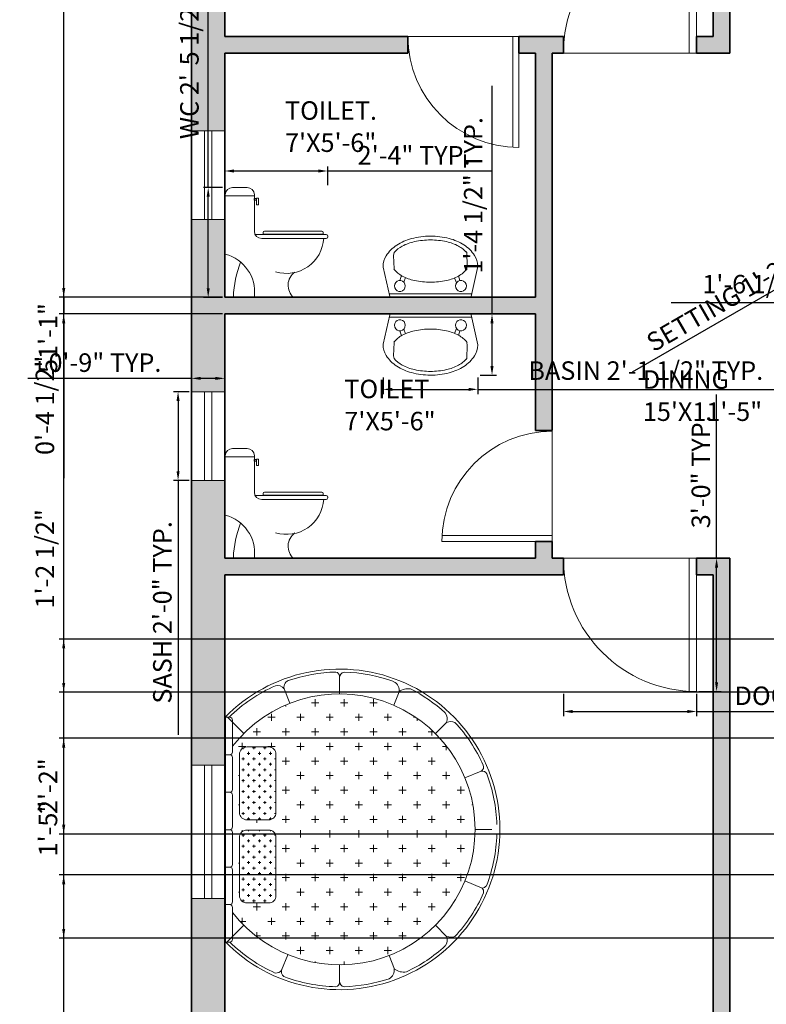
# Model space of a CAD drawing. Units: inches. Extents: x 2923 to 3500, y 1684 to 2381.
# Tile 2 of 12: x 2923 to 3125, y 1848 to 2114. Entities that reach past the tile are written whole.
import ezdxf

# ---------------------------------------------------------------- set-up
doc = ezdxf.new("R2010")
doc.units = ezdxf.units.IN
for name, color, linetype, lineweight in [('A-ANNO-DIMS', 2, 'Continuous', 18), ('A-AREA-IDEN', 7, 'Continuous', 18), ('A-DOOR', 3, 'Continuous', 18), ('A-FLOR-FIXT', 8, 'Continuous', 18), ('A-FURN-PATT', 8, 'Continuous', 13), ('A-GLAZ', 4, 'Continuous', 18), ('A-WALL', 7, 'Continuous', 35), ('A-WALL-PATT', 9, 'Continuous', 13), ('Furniture', 7, 'Continuous', 15)]:
    doc.layers.add(name, color=color, linetype=linetype, lineweight=lineweight)
doc.styles.get("Standard").update_dxf_attribs({"font": 'txt', "height": 5})
doc.dimstyles.new('ISO-25', dxfattribs={"dimtxt": 5, "dimasz": 2.5, "dimexe": 1.25, "dimexo": 0.625, "dimtad": 1, "dimlunit": 3, "dimtxsty": 'Standard', "dimcen": 2.5, "dimadec": 0, "dimazin": 0, "dimtfac": 1, "dimtmove": 0, "dimatfit": 3, "dimfxl": 1, "dimarcsym": 0})

# ---------------------------------------------------------------- blocks, each defined once
blk = doc.blocks.new('DOOR-SINGLE-36IN')
for p, q in [((36, 36), (0, 36)), ((34, 0.06), (34, 36)), ((36, 0), (36, 36))]:
    blk.add_line(p, q)
blk.add_arc((36, 36), 36, 180, 270)
blk = doc.blocks.new('DOOR-SINGLE-30IN')
for p, q in [((0, 30), (0, 0)), ((1.67, 29.95), (1.67, 0)), ((0, 0), (30, 0))]:
    blk.add_line(p, q)
blk.add_arc((0, 0), 30, 0, 90)
blk = doc.blocks.new('WINDOW-36IN')
for p, q in [((36, 9), (0, 9)), ((0, 9), (0, 0)), ((36, 0), (36, 9)), ((36, 5.5), (0, 5.5)), ((36, 3.5), (0, 3.5)), ((0, 0), (36, 0))]:
    blk.add_line(p, q)
blk = doc.blocks.new('WINDOW-24IN')
for p, q in [((9, 24), (0, 24)), ((0, 24), (0, 0)), ((3.5, 0), (3.5, 24)), ((5.5, 0), (5.5, 24)), ((9, 0), (9, 24)), ((0, 0), (9, 0))]:
    blk.add_line(p, q)
blk = doc.blocks.new('WC-FLOOR-MOUNT')
for p, q in [((6.05, 29.7), (2.11, 29.7)), ((0, 27.6), (0, 11.63)), ((7.97, 27.41), (0.2, 27.41)), ((8.49, 26.69), (7.97, 26.69)), ((7.97, 26.69), (7.97, 26.28)), ((8.02, 27.73), (8.02, 17.89)), ((8.02, 26.69), (8.02, 26.28)), ((8.49, 26.28), (8.49, 26.69)), ((9.1, 26.79), (8.59, 26.79)), ((8.59, 26.79), (8.59, 25.06)), ((9.1, 25.06), (9.1, 26.79)), ((7.97, 26.28), (8.49, 26.28)), ((8.59, 25.06), (9.1, 25.06)), ((27.42, 16.99), (8.24, 16.99)), ((10.4, 17.5), (10.4, 17.11)), ((10.4, 17.11), (26.62, 17.11)), ((26.23, 17.89), (10.79, 17.89)), ((15.89, 17.11), (15.89, 16.99)), ((23.77, 17.11), (23.77, 16.99)), ((26.62, 17.11), (26.62, 17.5)), ((27.82, 16.6), (27.82, 16.32)), ((27.42, 15.92), (9.99, 15.92)), ((8.02, 2.66), (8.02, 0.17)), ((8.02, 2.66), (8.02, 0.17)), ((18.71, 0.04), (2.25, 0.04))]:
    blk.add_line(p, q)
for centre, radius, start, end in [((2.11, 27.73), 1.97, 90, 180), ((6.05, 27.73), 1.97, 0, 90), ((9.99, 17.89), 1.97, 180, 270), ((10.79, 17.5), 0.394, 90, 180), ((16.71, 16.55), 10.05, 252.943, 356.7365), ((26.23, 17.5), 0.394, 0, 90), ((27.42, 16.6), 0.394, 0, 90), ((27.42, 16.32), 0.394, 270, 0), ((-2.41, 1.48), 10.5, 353.9182, 75.9043), ((31.43, -1.03), 29.12, 158.693, 177.6281), ((21.51, 3.3), 4.38, 125.5613, 228.8008)]:
    blk.add_arc(centre, radius, start, end)
blk = doc.blocks.new('BASIN-WALL-MOUNT')
for p, q in [((0, 8.4), (1.8, 16.33)), ((1.8, 16.54), (23.79, 16.54)), ((1.8, 16.13), (1.8, 16.54)), ((23.79, 16.54), (23.79, 16.13)), ((25.59, 8.23), (23.79, 16.33)), ((23.79, 15.64), (1.8, 15.64)), ((3.16, 14), (3.07, 13.48)), ((3.07, 13.48), (3.16, 12.95)), ((3.42, 14.46), (3.16, 14)), ((3.81, 14.8), (3.42, 14.46)), ((4.29, 14.98), (3.81, 14.8)), ((4.8, 14.98), (4.29, 14.98)), ((5.28, 14.8), (4.8, 14.98)), ((5.67, 14.46), (5.28, 14.8)), ((5.93, 14), (5.67, 14.46)), ((6.02, 13.48), (5.93, 14)), ((5.93, 12.95), (6.02, 13.48)), ((19.66, 14), (19.57, 13.48)), ((19.57, 13.48), (19.66, 12.95)), ((19.92, 14.46), (19.66, 14)), ((20.31, 14.8), (19.92, 14.46)), ((20.79, 14.98), (20.31, 14.8)), ((21.3, 14.98), (20.79, 14.98)), ((21.78, 14.8), (21.3, 14.98)), ((22.17, 14.46), (21.78, 14.8)), ((22.43, 14), (22.17, 14.46)), ((22.52, 13.48), (22.43, 14)), ((22.43, 12.95), (22.52, 13.48)), ((3.16, 12.95), (3.42, 12.49)), ((3.42, 12.49), (3.81, 12.15)), ((3.81, 12.15), (4.29, 11.97)), ((4.29, 11.97), (4.8, 11.97)), ((4.57, 11.96), (5.01, 10.67)), ((4.8, 11.97), (5.28, 12.15)), ((5.28, 12.15), (5.67, 12.49)), ((5.62, 12.45), (6.09, 11.17)), ((5.67, 12.49), (5.93, 12.95)), ((19.86, 12.63), (19.34, 11.26)), ((19.66, 12.95), (19.92, 12.49)), ((19.92, 12.49), (20.31, 12.15)), ((20.31, 12.15), (20.79, 11.97)), ((20.73, 11.97), (20.4, 10.75)), ((20.79, 11.97), (21.3, 11.97)), ((21.3, 11.97), (21.78, 12.15)), ((21.78, 12.15), (22.17, 12.49)), ((22.17, 12.49), (22.43, 12.95)), ((2.96, 8.83), (2.86, 5.21)), ((2.97, 8.99), (2.96, 8.98)), ((2.96, 8.98), (2.96, 8.97)), ((2.96, 8.97), (2.96, 8.96)), ((2.96, 8.83), (2.96, 8.96)), ((3.06, 9.08), (2.97, 8.99)), ((22.6, 4.46), (22.76, 8.08)), ((22.76, 8.08), (22.64, 8.8)), ((2.86, 5.21), (2.99, 4.47)), ((3.04, 4.25), (3.04, 4.25)), ((22.54, 4.2), (22.57, 4.35))]:
    blk.add_line(p, q)
for centre, radius, start, end in [((8.91, 3.89), 7.83, 118.2302, 139.6822), ((11.35, -0.82), 13.14, 102.6999, 117.8694), ((12.88, -8.38), 20.85, 90.2298, 102.2344), ((12.71, -8.38), 20.85, 77.7656, 89.7702), ((14.24, -0.82), 13.14, 62.1306, 77.3001), ((16.68, 3.89), 7.83, 39.3299, 61.7657), ((5.18, 8.21), 5.18, 177.9266, 179.8113), ((5.16, 8.15), 5.16, 179.1785, 213.1413), ((20.43, 8.08), 5.16, 326.4084, 0.3713), ((20.42, 8.14), 5.18, 359.7541, 0.9471), ((8.97, 10.54), 9.66, 212.6461, 237.0936), ((8.91, 9.59), 7.83, 220.8964, 241.7723), ((11.35, 14.31), 13.14, 242.1306, 257.3001), ((14.24, 14.31), 13.14, 282.6999, 297.8694), ((16.68, 9.59), 7.83, 298.2281, 319.1983), ((16.64, 10.51), 9.66, 302.4413, 326.8887), ((11.42, 14.45), 14.27, 237.383, 254.6821), ((12.95, 20.75), 20.75, 255.1956, 269.4863), ((12.88, 21.87), 20.85, 257.7656, 269.7702), ((12.75, 20.75), 20.75, 270.0316, 284.3223), ((12.71, 21.87), 20.85, 270.2298, 282.2344), ((14.23, 14.44), 14.27, 284.841, 302.14)]:
    blk.add_arc(centre, radius, start, end)
blk = doc.blocks.new('BED-ROUND-FRAME')
for p, q in [((31.04, 79.92), (31.04, 84.58)), ((31.04, 79.92), (31.04, 84.58)), ((17.61, 77.37), (16.05, 81.29)), ((45.66, 76.84), (47.11, 80.49)), ((0, 13.11), (0, 73.51)), ((5.15, 69.2), (0.74, 73.61)), ((5.15, 69.2), (0.74, 73.61)), ((56.93, 69.2), (59.95, 72.21)), ((56.93, 69.2), (59.95, 72.21)), ((59.95, 72.21), (56.93, 69.2)), ((13.83, 63.84), (13.83, 47.62)), ((64.9, 57.24), (69.31, 59.05)), ((69.31, 59.05), (69.4, 59.09)), ((67.65, 43.31), (72.18, 43.31)), ((13.83, 41.4), (13.83, 25.18)), ((13.83, 39.13), (13.84, 39.12)), ((64.9, 29.37), (69.53, 27.47)), ((0.42, 12.68), (5.15, 17.42)), ((0.42, 12.68), (5.15, 17.42)), ((59.95, 14.4), (56.93, 17.42)), ((17.07, 9.46), (15.35, 5.25)), ((44.42, 9.23), (45.86, 5.58)), ((31.04, 1.98), (31.04, 6.69)), ((31.04, 2.04), (31.04, 6.69))]:
    blk.add_line(p, q)
for points in [[(4, 47.85), (4, 63.6, -0.414214), (5.97, 65.57), (11.88, 65.57, -0.414214), (13.84, 63.6), (13.84, 47.85, -0.414214), (11.88, 45.89), (5.97, 45.89, -0.414214)], [(4, 25.41), (4, 41.16, -0.414214), (5.97, 43.13), (11.88, 43.13, -0.414214), (13.84, 41.16), (13.84, 25.41, -0.414214), (11.88, 23.45), (5.97, 23.45, -0.414214)]]:
    blk.add_lwpolyline(points, format="xyb", close=True)
for centre, radius, start, end in [((31.04, 43.31), 43.31, 224.213, 135.787), ((31.04, 43.31), 42.52, 91.3819, 109.0292), ((29.76, 84.56), 1.29, 359.0498, 78.348), ((32.5, 84.36), 1.46, 98.688, 183.9778), ((31.04, 43.31), 42.52, 69.8397, 88.3303), ((17.88, 81.76), 1.88, 111.9527, 202.5488), ((44.67, 80.98), 2.46, 345.7709, 65.4979), ((31.04, 43.31), 42.52, 114.0695, 134.5949), ((31.04, 43.31), 36.61, 217.8198, 142.1802), ((14.23, 79.9), 2.29, 37.3562, 103.3498), ((49.64, 77.03), 4.29, 82.908, 126.1659), ((31.04, 43.31), 42.52, 47.802, 63.2705), ((57.53, 73.21), 2.61, 337.5919, 37.6583), ((61.1, 69.09), 3.33, 70.4217, 110.1689), ((31.04, 43.31), 42.52, 24.0703, 42.854), ((69.6, 57.73), 1.36, 26.1665, 102.6069), ((68.6, 60.18), 1.35, 304.4266, 20.4145), ((31.04, 43.31), 42.52, 1.7281, 20.7271), ((31.04, 43.31), 42.52, 339.0428, 358.2719), ((69.4, 29.21), 1.75, 274.2316, 320.4352), ((68.35, 26.36), 1.62, 353.6066, 43.1756), ((31.04, 43.31), 42.52, 317.146, 336.245), ((57.53, 13.4), 2.61, 322.3417, 22.4081), ((61.1, 17.52), 3.33, 249.8311, 289.5783), ((31.04, 43.31), 42.52, 225.7269, 245.8957), ((31.04, 43.31), 42.52, 295.113, 312.198), ((16.89, 4.85), 1.59, 153.9459, 235.5493), ((42.79, 5.51), 3.04, 302.4304, 3.4261), ((48.39, 9.04), 4.29, 233.8341, 279.2916), ((13.85, 6.32), 1.83, 264.4179, 326.0029), ((31.04, 43.31), 42.52, 249.2703, 268.6181), ((31.04, 43.31), 42.52, 271.6697, 288.3347), ((29.76, 2.06), 1.29, 281.652, 0.9502), ((32.5, 2.25), 1.46, 176.0222, 261.312)]:
    blk.add_arc(centre, radius, start, end)
blk = doc.blocks.new('*D23')
at = {"layer": 'A-ANNO-DIMS', "color": 0, "lineweight": -2, "transparency": 16777216}
for p, q in [((2968.6, 2013.41), (2964.38, 2013.41)), ((2965.63, 2010.91), (2965.63, 1991.91)), ((2968.6, 1989.41), (2964.38, 1989.41)), ((2965.63, 1989.41), (2965.63, 1920.66))]:
    blk.add_line(p, q, dxfattribs=at)
at = {"layer": 'A-ANNO-DIMS', "color": 0, "transparency": 16777216}
for points in [[(2965.21, 2010.91), (2966.05, 2010.91), (2965.63, 2013.41)], [(2965.21, 1991.91), (2966.05, 1991.91), (2965.63, 1989.41)]]:
    blk.add_solid(points, dxfattribs=at)
at = {"layer": 'Defpoints', "color": 0, "transparency": 16777216}
for p in [(2969.23, 2013.41), (2965.63, 1989.41), (2969.23, 1989.41)]:
    blk.add_point(p, dxfattribs=at)
at = {"layer": 'A-ANNO-DIMS', "color": 0, "transparency": 16777216, "insert": (2962.03, 1953.78), "char_height": 5, "attachment_point": 5, "rotation": 90}
blk.add_mtext('SASH 2\'-0" TYP.', dxfattribs=at)
blk = doc.blocks.new('*D24')
at = {"layer": 'A-ANNO-DIMS', "color": 0, "lineweight": -2, "transparency": 16777216}
for p, q in [((2969.23, 2017.01), (2925, 2017.01)), ((2969.23, 2014.03), (2969.23, 2018.26)), ((2975.73, 2017.01), (2971.73, 2017.01)), ((2978.23, 2014.03), (2978.23, 2018.26))]:
    blk.add_line(p, q, dxfattribs=at)
at = {"layer": 'A-ANNO-DIMS', "color": 0, "transparency": 16777216}
for points in [[(2971.73, 2017.42), (2971.73, 2016.59), (2969.23, 2017.01)], [(2975.73, 2017.42), (2975.73, 2016.59), (2978.23, 2017.01)]]:
    blk.add_solid(points, dxfattribs=at)
at = {"layer": 'Defpoints', "color": 0, "transparency": 16777216}
for p in [(2969.23, 2017.01), (2969.23, 2013.41), (2978.23, 2013.41)]:
    blk.add_point(p, dxfattribs=at)
at = {"layer": 'A-ANNO-DIMS', "color": 0, "transparency": 16777216, "insert": (2945.87, 2020.61), "char_height": 5, "attachment_point": 5}
blk.add_mtext('0\'-9" TYP.', dxfattribs=at)
blk = doc.blocks.new('*D25')
at = {"layer": 'A-ANNO-DIMS', "color": 0, "lineweight": -2, "transparency": 16777216}
for p, q in [((3069.73, 1931.78), (3069.73, 1925.76)), ((3105.73, 1931.78), (3105.73, 1925.76)), ((3072.23, 1927.01), (3103.23, 1927.01)), ((3105.73, 1927.01), (3174.96, 1927.01))]:
    blk.add_line(p, q, dxfattribs=at)
at = {"layer": 'A-ANNO-DIMS', "color": 0, "transparency": 16777216}
for points in [[(3072.23, 1927.42), (3072.23, 1926.59), (3069.73, 1927.01)], [(3103.23, 1927.42), (3103.23, 1926.59), (3105.73, 1927.01)]]:
    blk.add_solid(points, dxfattribs=at)
at = {"layer": 'Defpoints', "color": 0, "transparency": 16777216}
for p in [(3069.73, 1932.41), (3105.73, 1932.41), (3105.73, 1927.01)]:
    blk.add_point(p, dxfattribs=at)
at = {"layer": 'A-ANNO-DIMS', "color": 0, "transparency": 16777216, "insert": (3141.59, 1930.61), "char_height": 5, "attachment_point": 5}
blk.add_mtext('DOOR 3\'-0" TYP.', dxfattribs=at)
blk = doc.blocks.new('*D26')
at = {"layer": 'A-ANNO-DIMS', "color": 0, "lineweight": -2, "transparency": 16777216}
for p, q in [((3111.13, 1968.41), (3111.13, 2012.63)), ((3106.35, 1968.41), (3112.38, 1968.41)), ((3111.13, 1934.91), (3111.13, 1965.91)), ((3106.35, 1932.41), (3112.38, 1932.41))]:
    blk.add_line(p, q, dxfattribs=at)
at = {"layer": 'A-ANNO-DIMS', "color": 0, "transparency": 16777216}
for points in [[(3110.71, 1965.91), (3111.55, 1965.91), (3111.13, 1968.41)], [(3110.71, 1934.91), (3111.55, 1934.91), (3111.13, 1932.41)]]:
    blk.add_solid(points, dxfattribs=at)
at = {"layer": 'Defpoints', "color": 0, "transparency": 16777216}
for p in [(3105.73, 1968.41), (3111.13, 1968.41), (3105.73, 1932.41)]:
    blk.add_point(p, dxfattribs=at)
at = {"layer": 'A-ANNO-DIMS', "color": 0, "transparency": 16777216, "insert": (3107.53, 1991.77), "char_height": 5, "attachment_point": 5, "rotation": 90}
blk.add_mtext('3\'-0" TYP.', dxfattribs=at)
blk = doc.blocks.new('*D35')
at = {"layer": 'A-ANNO-DIMS', "color": 0, "lineweight": -2, "transparency": 16777216}
for p, q in [((2973.77, 2068.57), (2973.77, 2146.37)), ((2977.6, 2068.57), (2972.52, 2068.57)), ((2973.77, 2041.37), (2973.77, 2066.07)), ((2977.6, 2038.87), (2972.52, 2038.87))]:
    blk.add_line(p, q, dxfattribs=at)
at = {"layer": 'A-ANNO-DIMS', "color": 0, "transparency": 16777216}
for points in [[(2973.36, 2066.07), (2974.19, 2066.07), (2973.77, 2068.57)], [(2973.36, 2041.37), (2974.19, 2041.37), (2973.77, 2038.87)]]:
    blk.add_solid(points, dxfattribs=at)
at = {"layer": 'Defpoints', "color": 0, "transparency": 16777216}
for p in [(2973.77, 2068.57), (2978.23, 2068.57), (2978.23, 2038.87)]:
    blk.add_point(p, dxfattribs=at)
at = {"layer": 'A-ANNO-DIMS', "color": 0, "transparency": 16777216, "insert": (2969.34, 2108.72), "char_height": 5, "attachment_point": 5, "rotation": 90}
blk.add_mtext('WC 2\'-5 1/2" TYP.', dxfattribs=at)
blk = doc.blocks.new('*D36')
at = {"layer": 'A-ANNO-DIMS', "color": 0, "lineweight": -2, "transparency": 16777216}
for p, q in [((2978.23, 2069.2), (2978.23, 2074.28)), ((2980.73, 2073.03), (3003.55, 2073.03)), ((3006.05, 2069.2), (3006.05, 2074.28)), ((3006.05, 2073.03), (3050.27, 2073.03))]:
    blk.add_line(p, q, dxfattribs=at)
at = {"layer": 'A-ANNO-DIMS', "color": 0, "transparency": 16777216}
for points in [[(2980.73, 2073.44), (2980.73, 2072.61), (2978.23, 2073.03)], [(3003.55, 2073.44), (3003.55, 2072.61), (3006.05, 2073.03)]]:
    blk.add_solid(points, dxfattribs=at)
at = {"layer": 'Defpoints', "color": 0, "transparency": 16777216}
for p in [(3006.05, 2073.03), (2978.23, 2068.57), (3006.05, 2068.57)]:
    blk.add_point(p, dxfattribs=at)
at = {"layer": 'A-ANNO-DIMS', "color": 0, "transparency": 16777216, "insert": (3029.41, 2076.63), "char_height": 5, "attachment_point": 5}
blk.add_mtext('2\'-4" TYP.', dxfattribs=at)
blk = doc.blocks.new('*D37')
at = {"layer": 'A-ANNO-DIMS', "color": 0, "lineweight": -2, "transparency": 16777216}
for p, q in [((3021, 2017.25), (3021, 2012.78)), ((3046.61, 2017.25), (3046.61, 2012.78)), ((3023.5, 2014.03), (3044.11, 2014.03)), ((3046.61, 2014.03), (3134.88, 2014.03))]:
    blk.add_line(p, q, dxfattribs=at)
at = {"layer": 'A-ANNO-DIMS', "color": 0, "transparency": 16777216}
for points in [[(3023.5, 2014.45), (3023.5, 2013.61), (3021, 2014.03)], [(3044.11, 2014.45), (3044.11, 2013.61), (3046.61, 2014.03)]]:
    blk.add_solid(points, dxfattribs=at)
at = {"layer": 'Defpoints', "color": 0, "transparency": 16777216}
for p in [(3021, 2017.87), (3046.61, 2017.87), (3046.61, 2014.03)]:
    blk.add_point(p, dxfattribs=at)
at = {"layer": 'A-ANNO-DIMS', "color": 0, "transparency": 16777216, "insert": (3092, 2018.46), "char_height": 5, "attachment_point": 5}
blk.add_mtext('BASIN 2\'-1 1/2" TYP.', dxfattribs=at)
blk = doc.blocks.new('*D38')
at = {"layer": 'A-ANNO-DIMS', "color": 0, "lineweight": -2, "transparency": 16777216}
for p, q in [((3050.45, 2034.41), (3050.45, 2096.01)), ((3047.23, 2034.41), (3051.7, 2034.41)), ((3050.45, 2020.37), (3050.45, 2031.91)), ((3047.23, 2017.87), (3051.7, 2017.87))]:
    blk.add_line(p, q, dxfattribs=at)
at = {"layer": 'A-ANNO-DIMS', "color": 0, "transparency": 16777216}
for points in [[(3050.03, 2031.91), (3050.87, 2031.91), (3050.45, 2034.41)], [(3050.03, 2020.37), (3050.87, 2020.37), (3050.45, 2017.87)]]:
    blk.add_solid(points, dxfattribs=at)
at = {"layer": 'Defpoints', "color": 0, "transparency": 16777216}
for p in [(3046.61, 2034.41), (3050.45, 2034.41), (3046.61, 2017.87)]:
    blk.add_point(p, dxfattribs=at)
at = {"layer": 'A-ANNO-DIMS', "color": 0, "transparency": 16777216, "insert": (3046.02, 2066.46), "char_height": 5, "attachment_point": 5, "rotation": 90}
blk.add_mtext('1\'-4 1/2" TYP.', dxfattribs=at)
blk = doc.blocks.new('*D40')
at = {"layer": 'A-ANNO-DIMS', "color": 0, "lineweight": -2, "transparency": 16777216}
for p, q in [((3160.47, 2034.91), (3160.47, 2038.63)), ((3178.95, 2034.91), (3178.95, 2038.63)), ((3160.47, 2037.38), (3098.86, 2037.38)), ((3176.45, 2037.38), (3162.97, 2037.38))]:
    blk.add_line(p, q, dxfattribs=at)
at = {"layer": 'A-ANNO-DIMS', "color": 0, "transparency": 16777216}
for points in [[(3162.97, 2037.8), (3162.97, 2036.96), (3160.47, 2037.38)], [(3176.45, 2037.8), (3176.45, 2036.96), (3178.95, 2037.38)]]:
    blk.add_solid(points, dxfattribs=at)
at = {"layer": 'Defpoints', "color": 0, "transparency": 16777216}
for p in [(3160.47, 2037.38), (3160.47, 2034.29), (3178.95, 2034.29)]:
    blk.add_point(p, dxfattribs=at)
at = {"layer": 'A-ANNO-DIMS', "color": 0, "transparency": 16777216, "insert": (3128.42, 2041.81), "char_height": 5, "attachment_point": 5}
blk.add_mtext('1\'-6 1/2" TYP.', dxfattribs=at)
blk = doc.blocks.new('*D41')
at = {"layer": 'A-ANNO-DIMS', "color": 0, "lineweight": -2, "transparency": 16777216}
for p, q in [((3166.89, 2065.67), (3168.23, 2063.34)), ((3165.44, 2063.18), (3157.85, 2058.8)), ((3155.69, 2057.55), (3088.31, 2018.65)), ((3154.97, 2058.79), (3156.31, 2056.46))]:
    blk.add_line(p, q, dxfattribs=at)
at = {"layer": 'A-ANNO-DIMS', "color": 0, "transparency": 16777216}
for points in [[(3165.23, 2063.54), (3165.65, 2062.82), (3167.61, 2064.43)], [(3157.64, 2059.16), (3158.06, 2058.43), (3155.69, 2057.55)]]:
    blk.add_solid(points, dxfattribs=at)
at = {"layer": 'Defpoints', "color": 0, "transparency": 16777216}
for p in [(3166.57, 2066.21), (3154.66, 2059.33), (3155.69, 2057.55)]:
    blk.add_point(p, dxfattribs=at)
at = {"layer": 'A-ANNO-DIMS', "color": 0, "transparency": 16777216, "insert": (3119.12, 2040.59), "char_height": 5, "attachment_point": 5, "rotation": 30}
blk.add_mtext('SETTING 1\'-2" TYP.', dxfattribs=at)
blk = doc.blocks.new('*D49')
at = {"layer": 'A-ANNO-DIMS', "color": 0, "lineweight": -2, "transparency": 16777216}
for p, q in [((2969.23, 2263.03), (2969.23, 2370.16)), ((3444.23, 2110.03), (3444.23, 2370.16)), ((2971.73, 2368.91), (3441.73, 2368.91))]:
    blk.add_line(p, q, dxfattribs=at)
at = {"layer": 'A-ANNO-DIMS', "color": 0, "transparency": 16777216}
for points in [[(2971.73, 2369.32), (2971.73, 2368.49), (2969.23, 2368.91)], [(3441.73, 2369.32), (3441.73, 2368.49), (3444.23, 2368.91)]]:
    blk.add_solid(points, dxfattribs=at)
at = {"layer": 'Defpoints', "color": 0, "transparency": 16777216}
for p in [(3444.23, 2368.91), (2969.23, 2262.41), (3444.23, 2109.41)]:
    blk.add_point(p, dxfattribs=at)
at = {"layer": 'A-ANNO-DIMS', "color": 0, "transparency": 16777216, "insert": (3206.73, 2372.51), "char_height": 5, "attachment_point": 5}
blk.add_mtext('39\'-7"', dxfattribs=at)
blk = doc.blocks.new('*D50')
at = {"layer": 'A-ANNO-DIMS', "color": 0, "lineweight": -2, "transparency": 16777216}
for p, q in [((2991.1, 2334.41), (2933.48, 2334.41)), ((2934.73, 1723.91), (2934.73, 2331.91)), ((3109.6, 1721.41), (2933.48, 1721.41))]:
    blk.add_line(p, q, dxfattribs=at)
at = {"layer": 'A-ANNO-DIMS', "color": 0, "transparency": 16777216}
for points in [[(2934.31, 2331.91), (2935.15, 2331.91), (2934.73, 2334.41)], [(2934.31, 1723.91), (2935.15, 1723.91), (2934.73, 1721.41)]]:
    blk.add_solid(points, dxfattribs=at)
at = {"layer": 'Defpoints', "color": 0, "transparency": 16777216}
for p in [(2934.73, 2334.41), (2991.73, 2334.41), (3110.23, 1721.41)]:
    blk.add_point(p, dxfattribs=at)
at = {"layer": 'A-ANNO-DIMS', "color": 0, "transparency": 16777216, "insert": (2931.13, 2027.91), "char_height": 5, "attachment_point": 5, "rotation": 90}
blk.add_mtext('51\'-1"', dxfattribs=at)
blk = doc.blocks.new('*D51')
at = {"layer": 'A-ANNO-DIMS', "color": 0, "lineweight": -2, "transparency": 16777216}
for p, q in [((2934.73, 2041.41), (2934.73, 2043.91)), ((2977.6, 2038.91), (2933.48, 2038.91)), ((2934.73, 2038.91), (2934.73, 2034.41)), ((2977.6, 2034.41), (2933.48, 2034.41)), ((2934.73, 2031.91), (2934.73, 1990.06))]:
    blk.add_line(p, q, dxfattribs=at)
at = {"layer": 'A-ANNO-DIMS', "color": 0, "transparency": 16777216}
for points in [[(2934.31, 2041.41), (2935.15, 2041.41), (2934.73, 2038.91)], [(2934.31, 2031.91), (2935.15, 2031.91), (2934.73, 2034.41)]]:
    blk.add_solid(points, dxfattribs=at)
at = {"layer": 'Defpoints', "color": 0, "transparency": 16777216}
for p in [(2978.23, 2038.91), (2934.73, 2034.41), (2978.23, 2034.41)]:
    blk.add_point(p, dxfattribs=at)
at = {"layer": 'A-ANNO-DIMS', "color": 0, "transparency": 16777216, "insert": (2930.3, 2009.73), "char_height": 5, "attachment_point": 5, "rotation": 90}
blk.add_mtext('0\'-4 1/2"', dxfattribs=at)
blk = doc.blocks.new('*D63')
at = {"layer": 'A-ANNO-DIMS', "color": 0, "lineweight": -2, "transparency": 16777216}
for p, q in [((3203.71, 1919.77), (2933.48, 1919.77)), ((2934.73, 1896.41), (2934.73, 1917.27)), ((3203.71, 1893.91), (2933.48, 1893.91))]:
    blk.add_line(p, q, dxfattribs=at)
at = {"layer": 'A-ANNO-DIMS', "color": 0, "transparency": 16777216}
for points in [[(2934.31, 1917.27), (2935.15, 1917.27), (2934.73, 1919.77)], [(2934.31, 1896.41), (2935.15, 1896.41), (2934.73, 1893.91)]]:
    blk.add_solid(points, dxfattribs=at)
at = {"layer": 'Defpoints', "color": 0, "transparency": 16777216}
for p in [(2934.73, 1919.77), (3204.33, 1919.77), (3204.33, 1893.91)]:
    blk.add_point(p, dxfattribs=at)
at = {"layer": 'A-ANNO-DIMS', "color": 0, "transparency": 16777216, "insert": (2931.13, 1906.84), "char_height": 5, "attachment_point": 5, "rotation": 90}
blk.add_mtext('2\'-2"', dxfattribs=at)
blk = doc.blocks.new('*D65')
at = {"layer": 'A-ANNO-DIMS', "color": 0, "lineweight": -2, "transparency": 16777216}
for p, q in [((2934.73, 1882.85), (2934.73, 1905.41)), ((3193.07, 1882.85), (2933.48, 1882.85)), ((2934.73, 1868.29), (2934.73, 1880.35)), ((3193.07, 1865.79), (2933.48, 1865.79))]:
    blk.add_line(p, q, dxfattribs=at)
at = {"layer": 'A-ANNO-DIMS', "color": 0, "transparency": 16777216}
for points in [[(2934.31, 1880.35), (2935.15, 1880.35), (2934.73, 1882.85)], [(2934.31, 1868.29), (2935.15, 1868.29), (2934.73, 1865.79)]]:
    blk.add_solid(points, dxfattribs=at)
at = {"layer": 'Defpoints', "color": 0, "transparency": 16777216}
for p in [(2934.73, 1882.85), (3193.7, 1882.85), (3193.7, 1865.79)]:
    blk.add_point(p, dxfattribs=at)
at = {"layer": 'A-ANNO-DIMS', "color": 0, "transparency": 16777216, "insert": (2931.13, 1895.38), "char_height": 5, "attachment_point": 5, "rotation": 90}
blk.add_mtext('1\'-5"', dxfattribs=at)
blk = doc.blocks.new('*D67')
at = {"layer": 'A-ANNO-DIMS', "color": 0, "lineweight": -2, "transparency": 16777216}
for p, q in [((2934.73, 1946.56), (2934.73, 1987.45)), ((3208.37, 1946.56), (2933.48, 1946.56)), ((2934.73, 1934.74), (2934.73, 1944.06)), ((3208.37, 1932.24), (2933.48, 1932.24))]:
    blk.add_line(p, q, dxfattribs=at)
at = {"layer": 'A-ANNO-DIMS', "color": 0, "transparency": 16777216}
for points in [[(2934.31, 1944.06), (2935.15, 1944.06), (2934.73, 1946.56)], [(2934.31, 1934.74), (2935.15, 1934.74), (2934.73, 1932.24)]]:
    blk.add_solid(points, dxfattribs=at)
at = {"layer": 'Defpoints', "color": 0, "transparency": 16777216}
for p in [(2934.73, 1946.56), (3209, 1946.56), (3209, 1932.24)]:
    blk.add_point(p, dxfattribs=at)
at = {"layer": 'A-ANNO-DIMS', "color": 0, "transparency": 16777216, "insert": (2930.3, 1968.26), "char_height": 5, "attachment_point": 5, "rotation": 90}
blk.add_mtext('1\'-2 1/2"', dxfattribs=at)

msp = doc.modelspace()

# ---------------------------------------------------------------- hatches: boundary and pattern name
at = {"layer": 'A-FURN-PATT'}
h = msp.add_hatch(dxfattribs=at)
h.set_pattern_fill('CROSS', color=256, scale=15.748, angle=180, style=0)
h.set_pattern_definition([(360, (1245.7636, 386.063), (3.937, -3.937), [1.9685, -5.9055]), (270, (1246.748, 387.0473), (-3.937, -3.937), [1.9685, -5.9055])])
h.paths.add_polyline_path([(2980.347, 1917.607), (2980.347, 1915.314), (2979.599, 1915.314, -0.4142136), (2980.347, 1914.565), (2980.347, 1905.193), (2979.599, 1905.193, -0.4142136), (2980.347, 1904.445), (2980.347, 1895.073), (2979.599, 1895.073, -0.4142136), (2980.347, 1894.325), (2980.347, 1884.952), (2979.599, 1884.952, -0.4142136), (2980.347, 1884.204), (2980.347, 1874.832), (2979.599, 1874.832, -0.4142136), (2980.347, 1874.084), (2980.347, 1872.705, 2.9191153)])
h.paths.add_polyline_path([(2992.074, 1877.263, -0.4142136), (2990.105, 1875.294), (2984.2, 1875.294, -0.4142136), (2982.231, 1877.263), (2982.231, 1893.011, -0.4142136), (2984.2, 1894.979), (2990.105, 1894.979, -0.4142136), (2992.074, 1893.011)], flags=16)
h.paths.add_polyline_path([(2992.074, 1899.703, -0.4142136), (2990.105, 1897.735), (2984.2, 1897.735, -0.4142136), (2982.231, 1899.703), (2982.231, 1915.451, -0.4142136), (2984.2, 1917.42), (2990.105, 1917.42, -0.4142136), (2992.074, 1915.451)], flags=16)
h = msp.add_hatch(dxfattribs=at)
h.set_pattern_fill('CROSS', color=256, scale=5.9055, angle=450, style=0)
h.set_pattern_definition([(90, (3722.8477, 1218.4861), (-1.476375, 1.476375), [0.7381875, -2.2145625]), (180, (3723.2168, 1218.8552), (-1.476375, -1.476375), [0.7381875, -2.2145625])])
h.paths.add_polyline_path([(2982.231, 1877.263, 0.4142136), (2984.2, 1875.294), (2990.105, 1875.294, 0.4142136), (2992.074, 1877.263), (2992.074, 1893.011, 0.4142136), (2990.105, 1894.979), (2984.2, 1894.979, 0.4142136), (2982.231, 1893.011)])
h.paths.add_polyline_path([(2992.074, 1915.451, 0.4142136), (2990.105, 1917.42), (2984.2, 1917.42, 0.4142136), (2982.231, 1915.451), (2982.231, 1899.703, 0.4142136), (2984.2, 1897.735), (2990.105, 1897.735, 0.4142136), (2992.074, 1899.703)])
at = {"layer": 'A-WALL-PATT'}
h = msp.add_hatch(color=256, dxfattribs=at)
h.dxf.hatch_style = 1
h.paths.add_polyline_path([(3014.23, 2262.406), (2969.23, 2262.406), (2969.23, 2201.5), (2978.23, 2201.5), (2978.23, 2213.699), (2978.23, 2253.406), (3014.23, 2253.406)])
h.paths.add_polyline_path([(3119.23, 2262.406), (3074.23, 2262.406), (3074.23, 2253.406), (3110.23, 2253.406), (3110.23, 2109.406), (3105.73, 2109.406), (3105.73, 2104.906), (3114.73, 2104.906), (3114.73, 2152.906), (3119.23, 2152.906), (3119.23, 2157.406), (3114.73, 2157.406), (3114.73, 2253.406), (3119.23, 2253.406)])
h.paths.add_polyline_path([(3179.98, 2262.406), (3149.23, 2262.406), (3149.23, 2253.406), (3179.98, 2253.406)], flags=0)
h.paths.add_polyline_path([(3295.73, 2262.406), (3215.98, 2262.406), (3215.98, 2253.406), (3246.73, 2253.406), (3246.73, 2157.406), (3149.23, 2157.406), (3149.23, 2152.906), (3246.73, 2152.906), (3246.73, 2149.906), (3251.23, 2149.906), (3251.23, 2253.406), (3295.73, 2253.406)])
h.paths.add_polyline_path([(3397.23, 2262.406), (3343.73, 2262.406), (3343.73, 2253.406), (3349.929, 2253.406), (3388.23, 2253.406), (3388.23, 2199.406), (3397.23, 2199.406)])
h.paths.add_polyline_path([(3369.935, 2334.406), (3264.935, 2334.406), (3264.935, 2262.406), (3269.435, 2262.406), (3269.435, 2329.906), (3365.435, 2329.906), (3365.435, 2262.406), (3369.935, 2262.406)])
h.paths.add_polyline_path([(3096.73, 2334.406), (2991.73, 2334.406), (2991.73, 2262.406), (2996.23, 2262.406), (2996.23, 2329.906), (3092.23, 2329.906), (3092.23, 2262.406), (3096.73, 2262.406)])
h.paths.add_polyline_path([(3397.23, 2163.406), (3388.23, 2163.406), (3388.23, 2109.406), (3251.23, 2109.406), (3251.23, 2113.906), (3246.73, 2113.906), (3246.73, 2092.906), (3251.23, 2092.906), (3251.23, 2104.906), (3435.23, 2104.906), (3435.23, 2080.906), (3444.23, 2080.906), (3444.23, 2109.406), (3397.23, 2109.406)])
h.paths.add_polyline_path([(3444.23, 2044.906), (3435.23, 2044.906), (3435.23, 2020.906), (3251.23, 2020.906), (3251.23, 2032.906), (3246.73, 2032.906), (3246.73, 2016.406), (3251.23, 2016.406), (3287.73, 2016.406), (3287.73, 1968.406), (3287.23, 1968.406), (3287.23, 1963.906), (3296.73, 1963.906), (3296.73, 1968.406), (3292.23, 1968.406), (3292.23, 2016.406), (3388.23, 2016.406), (3388.23, 2004.398), (3397.23, 2004.398), (3397.23, 2016.406), (3444.23, 2016.406)])
h.paths.add_polyline_path([(3397.23, 1980.398), (3388.23, 1980.398), (3388.23, 1979.998), (3388.23, 1969.828), (3388.23, 1968.406), (3326.73, 1968.406), (3326.73, 1963.906), (3388.23, 1963.906), (3388.23, 1913.156), (3397.23, 1913.156)])
h.paths.add_polyline_path([(3251.23, 1968.406), (3150.73, 1968.406), (3150.73, 1963.906), (3246.73, 1963.906), (3246.73, 1826.406), (3230.98, 1826.406), (3230.98, 1817.406), (3251.23, 1817.406), (3251.23, 1963.906)])
h.paths.add_polyline_path([(3114.73, 1968.406), (3105.73, 1968.406), (3105.73, 1963.906), (3110.23, 1963.906), (3110.23, 1817.406), (3119.23, 1817.406), (3119.23, 1826.406), (3114.73, 1826.406)])
h.paths.add_polyline_path([(3069.73, 1968.406), (3066.73, 1968.406), (3066.73, 1972.906), (3062.23, 1972.906), (3062.23, 1968.406), (2978.23, 1968.406), (2978.23, 1989.406), (2969.23, 1989.406), (2969.23, 1912.505), (2978.23, 1912.505), (2978.23, 1925.355), (2978.23, 1963.906), (3069.73, 1963.906)])
h.paths.add_polyline_path([(3066.73, 2104.906), (3069.73, 2104.906), (3069.73, 2109.406), (3057.73, 2109.406), (3057.73, 2104.906), (3062.23, 2104.906), (3062.23, 2038.906), (2978.23, 2038.906), (2978.23, 2059.906), (2969.23, 2059.906), (2969.23, 2013.406), (2978.23, 2013.406), (2978.23, 2034.406), (3062.23, 2034.406), (3062.23, 2002.906), (3066.73, 2002.906)])
h.paths.add_polyline_path([(3027.73, 2109.406), (2978.23, 2109.406), (2978.23, 2165.5), (2969.23, 2165.5), (2969.23, 2083.906), (2978.23, 2083.906), (2978.23, 2104.906), (3027.73, 2104.906)])
h.paths.add_polyline_path([(2978.23, 1876.505), (2969.23, 1876.505), (2969.23, 1817.406), (3014.23, 1817.406), (3014.23, 1826.406), (2978.23, 1826.406)])
h.paths.add_polyline_path([(2996.23, 1817.406), (2991.73, 1817.406), (2991.73, 1745.406), (3096.73, 1745.406), (3096.73, 1817.406), (3092.23, 1817.406), (3092.23, 1749.906), (2996.23, 1749.906)])
h.paths.add_polyline_path([(3289.73, 1826.406), (3251.23, 1826.406), (3251.23, 1817.406), (3289.73, 1817.406)])
h.paths.add_polyline_path([(3397.23, 1877.156), (3388.23, 1877.156), (3388.23, 1864.957), (3388.23, 1826.406), (3349.73, 1826.406), (3349.73, 1817.406), (3397.23, 1817.406)])
h.paths.add_polyline_path([(3374.267, 1817.406), (3369.767, 1817.406), (3369.767, 1749.906), (3273.767, 1749.906), (3273.767, 1817.406), (3269.267, 1817.406), (3269.267, 1745.406), (3374.267, 1745.406)])

# ---------------------------------------------------------------- linework, layer by layer
at = {"layer": 'A-DOOR'}
for p, q in [((3066.73, 1972.906), (3066.73, 2002.75)), ((3036.932, 1974.564), (3066.73, 1974.564)), ((3036.886, 1972.906), (3066.73, 1972.906))]:
    msp.add_line(p, q, dxfattribs=at)
msp.add_arc((3066.73, 1972.906), 29.844, 90, 180, dxfattribs=at)
at = {"layer": 'A-WALL'}
for p, q in [((2969.23, 1817.406), (2969.23, 2262.406)), ((2978.23, 2109.406), (2978.23, 2253.406)), ((3110.23, 2109.406), (3110.23, 2253.406)), ((3114.73, 2104.906), (3114.73, 2152.906)), ((2978.23, 2109.406), (3027.73, 2109.406)), ((3027.73, 2104.906), (3027.73, 2109.406)), ((3057.73, 2104.906), (3057.73, 2109.406)), ((3057.73, 2109.406), (3069.73, 2109.406)), ((3069.73, 2109.406), (3069.73, 2104.906)), ((3105.73, 2109.406), (3105.73, 2104.906)), ((3105.73, 2109.406), (3110.23, 2109.406)), ((2978.23, 2104.906), (3027.73, 2104.906)), ((2978.23, 2038.906), (2978.23, 2104.906)), ((3057.73, 2104.906), (3062.23, 2104.906)), ((3062.23, 2038.906), (3062.23, 2104.906)), ((3066.73, 2104.906), (3069.73, 2104.906)), ((3066.73, 2002.906), (3066.73, 2104.906)), ((3105.73, 2104.906), (3114.73, 2104.906)), ((2978.23, 2038.906), (3062.23, 2038.906)), ((2978.23, 2034.406), (3062.23, 2034.406)), ((2978.23, 1968.406), (2978.23, 2034.406)), ((3062.23, 2002.906), (3062.23, 2034.406)), ((3062.23, 2002.906), (3066.73, 2002.906)), ((3062.23, 1968.406), (3062.23, 1972.906)), ((3062.23, 1972.906), (3066.73, 1972.906)), ((3066.73, 1968.406), (3066.73, 1972.906)), ((2978.23, 1968.406), (3062.23, 1968.406)), ((3066.73, 1968.406), (3069.73, 1968.406)), ((3069.73, 1963.906), (3069.73, 1968.406)), ((3105.73, 1963.906), (3105.73, 1968.406)), ((3105.73, 1968.406), (3114.73, 1968.406)), ((3114.73, 1826.406), (3114.73, 1968.406)), ((2978.23, 1826.406), (2978.23, 1963.906)), ((2978.23, 1963.906), (3069.73, 1963.906)), ((3105.73, 1963.906), (3110.23, 1963.906)), ((3110.23, 1721.406), (3110.23, 1963.906))]:
    msp.add_line(p, q, dxfattribs=at)
at = {"layer": 'Furniture'}
for points in [[(2980.347, 1916.062), (2980.347, 1924.686, 0.4142136), (2979.599, 1925.434), (2978.458, 1925.434), (2978.458, 1915.314), (2979.599, 1915.314, 0.4142136)], [(2980.347, 1905.941), (2980.347, 1914.565, 0.4142136), (2979.599, 1915.314), (2978.458, 1915.314), (2978.458, 1905.193), (2979.599, 1905.193, 0.4142136)], [(2980.347, 1895.821), (2980.347, 1904.445, 0.4142136), (2979.599, 1905.193), (2978.458, 1905.193), (2978.458, 1895.073), (2979.599, 1895.073, 0.4142136)], [(2980.347, 1885.7), (2980.347, 1894.325, 0.4142136), (2979.599, 1895.073), (2978.458, 1895.073), (2978.458, 1884.952), (2979.599, 1884.952, 0.4142136)], [(2980.347, 1875.58), (2980.347, 1884.204, 0.4142136), (2979.599, 1884.952), (2978.458, 1884.952), (2978.458, 1874.832), (2979.599, 1874.832, 0.4142136)], [(2980.347, 1865.459), (2980.347, 1874.084, 0.4142136), (2979.599, 1874.832), (2978.458, 1874.832), (2978.458, 1864.711), (2979.599, 1864.711, 0.4142136)]]:
    msp.add_lwpolyline(points, format="xyb", close=True, dxfattribs=at)

# ---------------------------------------------------------------- block references
at = {"layer": 'A-DOOR', "extrusion": (0, 0, -1), "zscale": -1, "rotation": 180}
msp.add_blockref('DOOR-SINGLE-36IN', (-3069.73, 2140.906), dxfattribs=at)
at = {"layer": 'A-DOOR', "rotation": 180}
msp.add_blockref('DOOR-SINGLE-30IN', (3057.73, 2109.406), dxfattribs=at)
at = {"layer": 'A-DOOR'}
msp.add_blockref('DOOR-SINGLE-36IN', (3069.73, 1932.406), dxfattribs=at)
at = {"layer": 'A-FLOR-FIXT'}
for name, p in [('WC-FLOOR-MOUNT', (2978.23, 2038.87)), ('BASIN-WALL-MOUNT', (3021.012, 2017.871)), ('WC-FLOOR-MOUNT', (2978.23, 1968.37))]:
    msp.add_blockref(name, p, dxfattribs=at)
at = {"layer": 'A-FLOR-FIXT', "extrusion": (0, 0, -1), "zscale": -1, "rotation": 180}
msp.add_blockref('BASIN-WALL-MOUNT', (-3021.012, 2055.441), dxfattribs=at)
at = {"layer": 'A-GLAZ'}
msp.add_blockref('WINDOW-24IN', (2969.23, 2059.906), dxfattribs=at)
for name, p, rotation in [('WINDOW-24IN', (2978.23, 2013.406), 180), ('WINDOW-36IN', (2969.23, 1912.505), 269.9999999999973)]:
    msp.add_blockref(name, p, dxfattribs=dict(at, rotation=rotation))
at = {"layer": 'Furniture'}
msp.add_blockref('BED-ROUND-FRAME', (2978.23, 1851.849), dxfattribs=at)

# ---------------------------------------------------------------- texts
at = {"layer": 'A-AREA-IDEN'}
for s, p in [('TOILET.', (2994.525, 2086.866)), ('7\'X5\'-6"', (2994.525, 2078.181)), ('DINING', (3091.21, 2014.19)), ('TOILET', (3010.552, 2011.649)), ('15\'X11\'-5"', (3091.21, 2005.505)), ('7\'X5\'-6"', (3010.552, 2002.964))]:
    msp.add_text(s, height=5, dxfattribs=at).set_placement(p)

# ---------------------------------------------------------------- dimensions: what is measured, and where the dimension line sits
at = {"layer": 'A-ANNO-DIMS'}
dim = msp.add_linear_dim(base=(3444.23, 2368.906), p1=(2969.23, 2262.406), p2=(3444.23, 2109.406), dimstyle='ISO-25', override={"dimdec": 1, "dimlfac": 1, "dimrnd": 0, "dimzin": 1, "dimdsep": 46, "dimlunit": 4, "dimfrac": 2}, dxfattribs=at)
dim.commit()
dim.dimension.update_dxf_attribs({"geometry": '*D49', "text_midpoint": (3206.73, 2372.507)})
for base, p1, p2, picture, middle in [((2934.73, 2334.406), (3110.23, 1721.406), (2991.73, 2334.406), '*D50', (2931.129, 2027.906)), ((2934.73, 2034.406), (2978.23, 2038.906), (2978.23, 2034.406), '*D51', (2930.295, 2009.734)), ((2934.73, 1946.56), (3209, 1932.241), (3209, 1946.56), '*D67', (2930.295, 1968.256)), ((2934.73, 1919.766), (3204.334, 1893.912), (3204.334, 1919.766), '*D63', (2931.129, 1906.839)), ((2934.73, 1882.852), (3193.699, 1865.788), (3193.699, 1882.852), '*D65', (2931.129, 1895.382))]:
    dim = msp.add_linear_dim(base=base, p1=p1, p2=p2, angle=90, dimstyle='ISO-25', override={"dimdec": 1, "dimlfac": 1, "dimrnd": 0, "dimzin": 1, "dimdsep": 46, "dimlunit": 4, "dimfrac": 2}, dxfattribs=at)
    dim.commit()
    dim.dimension.update_dxf_attribs({"geometry": picture, "text_midpoint": middle})
for base, p1, p2, angle, text, picture, middle in [((2973.775, 2068.571), (2978.23, 2038.87), (2978.23, 2068.571), 90, 'WC <> TYP.', '*D35', (2969.34, 2108.72)), ((3050.451, 2034.406), (3046.609, 2017.871), (3046.609, 2034.406), 90, '<> TYP.', '*D38', (3046.017, 2066.46)), ((3155.688, 2057.545), (3166.574, 2066.214), (3154.656, 2059.333), 210, 'SETTING <> TYP.', '*D41', (3119.118, 2040.59)), ((3160.47, 2037.379), (3178.949, 2034.288), (3160.47, 2034.288), 180, '<> TYP.', '*D40', (3128.417, 2041.814)), ((2969.23, 2017.006), (2978.23, 2013.406), (2969.23, 2013.406), 180, '<> TYP.', '*D24', (2945.867, 2020.607)), ((2965.63, 1989.406), (2969.23, 2013.406), (2969.23, 1989.406), 270, 'SASH <> TYP.', '*D23', (2962.029, 1953.781)), ((3111.13, 1968.406), (3105.73, 1932.406), (3105.73, 1968.406), 90, '<> TYP.', '*D26', (3107.529, 1991.769))]:
    dim = msp.add_linear_dim(base=base, p1=p1, p2=p2, angle=angle, text=text, dimstyle='ISO-25', override={"dimdec": 1, "dimlfac": 1, "dimrnd": 0, "dimzin": 1, "dimdsep": 46, "dimlunit": 4, "dimfrac": 2}, dxfattribs=at)
    dim.commit()
    dim.dimension.update_dxf_attribs({"geometry": picture, "text_midpoint": middle})
for base, p1, p2, text, picture, middle in [((3006.046, 2073.026), (2978.23, 2068.571), (3006.046, 2068.571), '<> TYP.', '*D36', (3029.409, 2076.628)), ((3046.609, 2014.029), (3020.997, 2017.871), (3046.609, 2017.871), 'BASIN <> TYP.', '*D37', (3091.996, 2018.464)), ((3105.73, 1927.006), (3069.73, 1932.406), (3105.73, 1932.406), 'DOOR <> TYP.', '*D25', (3141.593, 1930.607))]:
    dim = msp.add_linear_dim(base=base, p1=p1, p2=p2, text=text, dimstyle='ISO-25', override={"dimdec": 1, "dimlfac": 1, "dimrnd": 0, "dimzin": 1, "dimdsep": 46, "dimlunit": 4, "dimfrac": 2}, dxfattribs=at)
    dim.commit()
    dim.dimension.update_dxf_attribs({"geometry": picture, "text_midpoint": middle})

doc.saveas('drawing.dxf')
